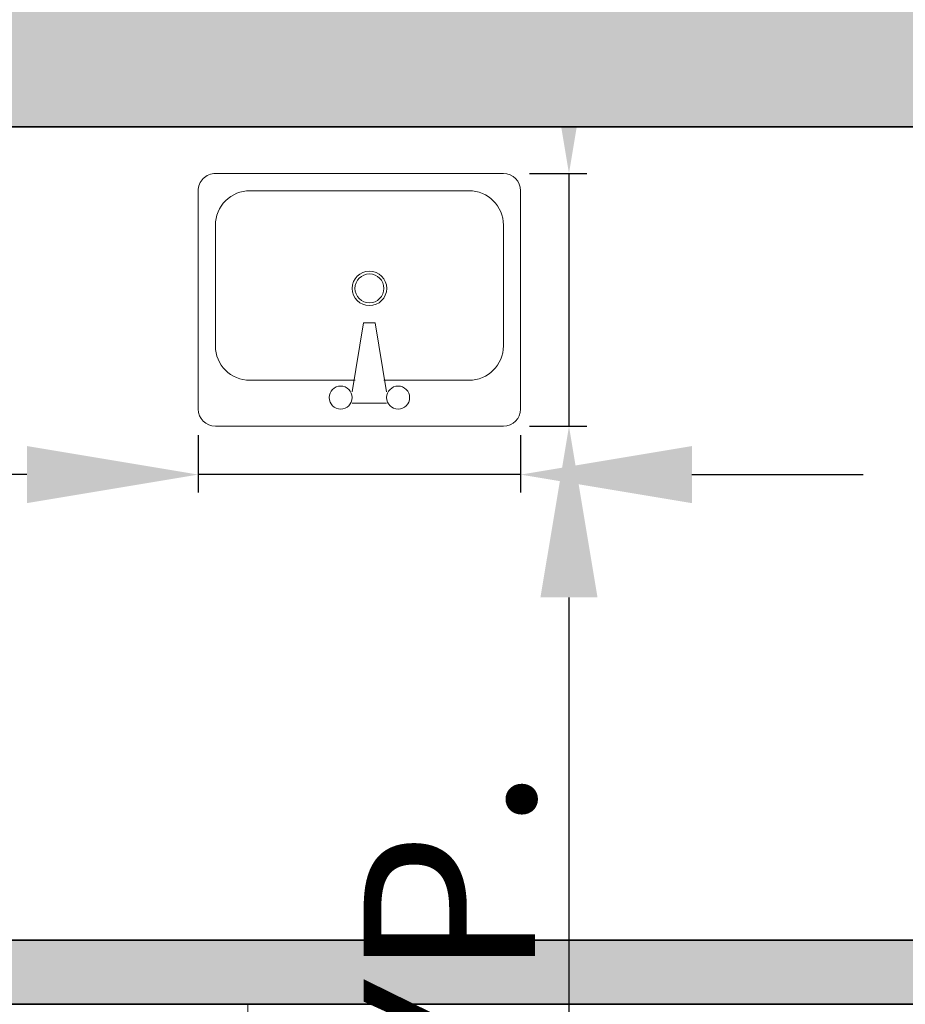
# Model space of a CAD drawing. Units: inches. Extents: x 2083 to 3317, y 1141 to 2115.
# Tile 247 of 256: x 3006 to 3068, y 1416 to 1485. Entities that reach past the tile are written whole.
import ezdxf

# ---------------------------------------------------------------- set-up
doc = ezdxf.new("R2010")
doc.units = ezdxf.units.IN
for name, color, linetype, lineweight in [('A-ANNO-DIMS', 2, 'Continuous', 18), ('A-FLOR-CASE', 8, 'Continuous', 18), ('A-FLOR-FIXT', 9, 'Continuous', 18), ('A-WALL', 7, 'Continuous', 35)]:
    doc.layers.add(name, color=color, linetype=linetype, lineweight=lineweight)
doc.layers.add('A-WALL-PATT', color=251, linetype='Continuous', lineweight=13, true_color=0x636466)
doc.styles.add('DIM_FONT', font='TXT.shx', dxfattribs={"width": 0.8})
doc.styles.get("Standard").update_dxf_attribs({"font": 'arial.ttf'})
doc.dimstyles.new('ISO-25', dxfattribs={"dimtxt": 12, "dimasz": 12, "dimexe": 1.25, "dimexo": 0.625, "dimtad": 1, "dimlunit": 3, "dimtxsty": 'Standard', "dimcen": 2.5, "dimadec": 0, "dimazin": 0, "dimtfac": 1, "dimtmove": 0, "dimatfit": 3, "dimfxl": 1, "dimarcsym": 0})

# ---------------------------------------------------------------- blocks, each defined once
blk = doc.blocks.new('A$C564A496C')
at = {"linetype": 'ByBlock'}
for p, q in [((543.2, 450), (30.7, 450)), ((0, 419.3), (0, 30.7)), ((238.5, 409.1), (299.8, 409.1)), ((573.8, 30.7), (573.8, 419.3)), ((238.5, 388.6), (258.9, 265.9)), ((279.4, 265.9), (299.8, 388.6)), ((92, 368.2), (243.6, 368.2)), ((294.7, 368.2), (481.8, 368.2)), ((30.7, 92), (30.7, 306.8)), ((543.2, 306.8), (543.2, 92)), ((258.9, 265.9), (279.4, 265.9)), ((481.8, 30.7), (92, 30.7)), ((30.7, 0), (543.2, 0))]:
    blk.add_line(p, q, dxfattribs=at)
for centre, radius in [((218, 398.9), 20.5), ((320.3, 398.9), 20.5), ((269.1, 204.5), 30.7), ((269.1, 204.5), 25.7)]:
    blk.add_circle(centre, radius, dxfattribs=at)
for centre, radius, start, end in [((30.7, 419.3), 30.7, 90, 180), ((543.2, 419.3), 30.7, 0, 90), ((92, 306.8), 61.4, 90, 180), ((481.8, 306.8), 61.4, 0, 90), ((92, 92), 61.4, 180, 270), ((481.8, 92), 61.4, 270, 0), ((30.7, 30.7), 30.7, 180, 270), ((543.2, 30.7), 30.7, 270, 0)]:
    blk.add_arc(centre, radius, start, end, dxfattribs=at)
at = {"style": 'DIM_FONT', "width": 0.8, "flags": 9}
for tag in ['YSIZE', 'XSIZE']:
    blk.add_attdef(tag, (269.1, 450), '', height=0.5, rotation=270, dxfattribs=at)
blk = doc.blocks.new('CASEWORK-96X24')
for q in [(0, 0), (24, 96)]:
    blk.add_line((0, 96), q)
blk = doc.blocks.new('*D18')
at = {"layer": 'A-ANNO-DIMS', "color": 0, "lineweight": -2, "transparency": 16777216}
for p, q in [((3018.476, 1456.156), (3018.476, 1452.142)), ((3041.068, 1456.156), (3041.068, 1452.142)), ((3006.476, 1453.392), (2828.361, 1453.392)), ((3041.068, 1453.392), (3018.476, 1453.392)), ((3053.068, 1453.392), (3065.068, 1453.392))]:
    blk.add_line(p, q, dxfattribs=at)
at = {"layer": 'A-ANNO-DIMS', "color": 0, "transparency": 16777216}
for points in [[(3006.476, 1455.392), (3006.476, 1451.392), (3018.476, 1453.392)], [(3053.068, 1455.392), (3053.068, 1451.392), (3041.068, 1453.392)]]:
    blk.add_solid(points, dxfattribs=at)
at = {"layer": 'Defpoints', "color": 0, "transparency": 16777216}
for p in [(3018.476, 1456.781), (3041.068, 1456.781), (3018.476, 1453.392)]:
    blk.add_point(p, dxfattribs=at)
at = {"layer": 'A-ANNO-DIMS', "color": 0, "transparency": 16777216, "insert": (2911.418, 1460.222), "char_height": 12, "attachment_point": 5}
blk.add_mtext('BASIN 1\'-10 1/2" TYP.', dxfattribs=at)
blk = doc.blocks.new('*D19')
at = {"layer": 'A-ANNO-DIMS', "color": 0, "lineweight": -2, "transparency": 16777216}
for p, q in [((3044.457, 1486.497), (3044.457, 1498.497)), ((3041.693, 1474.497), (3045.707, 1474.497)), ((3044.457, 1474.497), (3044.457, 1456.781)), ((3041.693, 1456.781), (3045.707, 1456.781)), ((3044.457, 1444.781), (3044.457, 1331.553))]:
    blk.add_line(p, q, dxfattribs=at)
at = {"layer": 'A-ANNO-DIMS', "color": 0, "transparency": 16777216}
for points in [[(3042.457, 1486.497), (3046.457, 1486.497), (3044.457, 1474.497)], [(3042.457, 1444.781), (3046.457, 1444.781), (3044.457, 1456.781)]]:
    blk.add_solid(points, dxfattribs=at)
at = {"layer": 'Defpoints', "color": 0, "transparency": 16777216}
for p in [(3041.068, 1474.497), (3041.068, 1456.781), (3044.457, 1456.781)]:
    blk.add_point(p, dxfattribs=at)
at = {"layer": 'A-ANNO-DIMS', "color": 0, "transparency": 16777216, "insert": (3037.627, 1382.167), "char_height": 12, "attachment_point": 5, "rotation": 90}
blk.add_mtext('1\'-5 1/2" TYP.', dxfattribs=at)

msp = doc.modelspace()

# ---------------------------------------------------------------- hatches: boundary and pattern name
at = {"layer": 'A-WALL-PATT'}
h = msp.add_hatch(color=256, dxfattribs=at)
h.dxf.hatch_style = 1
h.paths.add_polyline_path([(3126.96, 2020.761), (2748.96, 2020.761), (2604.96, 2020.761), (2226.96, 2020.761), (2226.96, 1702.761), (2466.96, 1702.761), (2466.96, 1582.761), (2418.96, 1582.761), (2418.96, 1477.761), (2226.96, 1477.761), (2226.96, 1263.261), (2544.96, 1263.261), (2544.96, 1411.761), (2604.96, 1411.761), (2685.96, 1411.761), (2685.96, 1420.761), (2604.96, 1420.761), (2604.96, 1573.761), (2604.96, 1702.761), (2604.96, 2011.761), (2748.96, 2011.761), (2748.96, 1702.761), (2862.96, 1702.761), (2862.96, 1621.761), (2871.96, 1621.761), (2871.96, 1702.761), (2883.96, 1702.761), (2883.96, 1706.939, -0.026459), (2883.96, 1711.761), (2757.96, 1711.761), (2757.96, 1807.761), (2787.96, 1807.761), (2787.96, 1812.261), (2757.96, 1812.261), (2757.96, 2011.761), (2877.96, 2011.761), (2877.96, 1812.261), (2847.96, 1812.261), (2847.96, 1807.761), (2889.836, 1807.761), (2889.836, 1812.261), (2882.46, 1812.261), (2882.46, 2011.761), (3117.96, 2011.761), (3117.96, 1812.261), (2937.836, 1812.261), (2937.836, 1807.761), (2995.71, 1807.761), (2995.71, 1796.118), (3000.21, 1796.118), (3000.21, 1807.761), (3117.96, 1807.761), (3117.96, 1711.761), (3000.21, 1711.761), (3000.21, 1760.118), (2998.573, 1760.118, -0.020711), (2995.71, 1760.118), (2995.71, 1711.761), (2931.96, 1711.761), (2931.96, 1702.761), (3126.96, 1702.761)])
h.paths.add_polyline_path([(2471.46, 2011.761), (2471.46, 1810.011), (2462.717, 1810.011), (2462.717, 1805.511), (2505.96, 1805.511), (2505.96, 1810.011), (2475.96, 1810.011), (2475.96, 2011.761), (2595.96, 2011.761), (2595.96, 1810.011), (2565.96, 1810.011), (2565.96, 1805.511), (2595.96, 1805.511), (2595.96, 1711.761), (2235.96, 1711.761), (2235.96, 1805.511), (2353.71, 1805.511), (2353.71, 1796.054), (2358.21, 1796.054), (2358.21, 1805.511), (2414.717, 1805.511), (2414.717, 1810.011), (2235.96, 1810.011), (2235.96, 2011.761)], flags=16)
h.paths.add_polyline_path([(2270.205, 1994.61), (2270.205, 1970.61), (2246.205, 1970.61), (2246.205, 1994.61)], flags=0)
edge = h.paths.add_edge_path(flags=0)
edge.add_ellipse((2332.027, 1899.798), major_axis=(-3.043, 3.043), ratio=0.168252, start_angle=-161.33217, end_angle=-156.30711, ccw=False)
edge.add_ellipse((2333.082, 1898.744), major_axis=(-1.055, 1.055), ratio=0.453532, start_angle=-123.37102, end_angle=-94.15911)
edge = h.paths.add_edge_path(flags=0)
edge.add_ellipse((2332.027, 1968.876), major_axis=(3.043, 3.043), ratio=0.168252, start_angle=18.66783, end_angle=23.69289)
edge.add_spline(control_points=[(2332.926, 1970.691), (2332.227, 1970.336), (2330.894, 1969.659), (2328.413, 1970.932), (2327.204, 1967.749), (2324.71, 1969.956), (2322.533, 1967.012), (2320.013, 1971.296), (2317.68, 1968.158), (2316.041, 1967.102), (2315.427, 1966.81)], knot_values=[0, 0, 0, 0, 2.267059, 4.324559, 6.685584, 8.878641, 11.121502, 14.300359, 17.755284, 19.732645, 19.732645, 19.732645, 19.732645], degree=3, periodic=0)
edge.add_ellipse((2332.027, 1968.876), major_axis=(3.043, 3.043), ratio=0.168252, start_angle=18.66783, end_angle=23.69289, ccw=False)
edge.add_ellipse((2333.082, 1969.931), major_axis=(1.055, 1.055), ratio=0.453532, start_angle=56.62898, end_angle=85.84089, ccw=False)
edge = h.paths.add_edge_path(flags=0)
edge.add_spline(control_points=[(2296.428, 1967.988), (2293.628, 1965.336), (2287.704, 1959.727), (2299.744, 1949.996), (2294.533, 1935.669), (2290.573, 1920.604), (2293.394, 1909.974), (2296.185, 1904.967)], knot_values=[0.099185, 0.099185, 0.099185, 0.099185, 0.345301, 0.619822, 0.982653, 1.386093, 1.810555, 1.810555, 1.810555, 1.810555], degree=3, periodic=0)
edge.add_spline(control_points=[(2296.185, 1904.967), (2297.384, 1902.619), (2298.001, 1901.949), (2298.553, 1901.468)], knot_values=[0.006246, 0.006246, 0.006246, 0.006246, 0.055476, 0.055476, 0.055476, 0.055476], degree=3, periodic=0)
edge.add_spline(control_points=[(2298.553, 1901.468), (2297.259, 1900.923), (2295.225, 1900.232), (2293.06, 1900.614), (2292.101, 1900.788), (2292.09, 1900.791)], knot_values=[0.312835, 0.312835, 0.312835, 0.312835, 0.40178, 0.474987, 0.475903, 0.475903, 0.475903, 0.475903], degree=3, periodic=0)
edge.add_arc((2292.794, 1904.664), 3.937, 215.4209, 259.69818, ccw=False)
edge.add_spline(control_points=[(2289.585, 1902.382), (2289.477, 1902.535), (2289.368, 1902.688), (2289.261, 1902.841)], knot_values=[0.102872, 0.102872, 0.102872, 0.102872, 0.116896, 0.116896, 0.116896, 0.116896], degree=3, periodic=0)
edge.add_spline(control_points=[(2289.261, 1902.841), (2288.687, 1902.55), (2287.64, 1902.02), (2285.881, 1901.874), (2283.853, 1901.504), (2281.72, 1899.711), (2278.467, 1899.493), (2276.157, 1901.883), (2272.259, 1899.804), (2267.778, 1901.843), (2262.244, 1900.184), (2257.415, 1901.782), (2254.318, 1900.726), (2253.178, 1900.337)], knot_values=[0, 0, 0, 0, 1.907977, 3.477176, 5.261074, 7.972851, 11.680248, 13.717921, 16.939592, 22.789562, 27.502503, 33.595215, 37.145618, 37.145618, 37.145618, 37.145618], degree=3, periodic=0)
edge.add_line((2253.178, 1900.337), (2250.244, 1902.841))
edge.add_line((2250.244, 1902.841), (2250.244, 1965.833))
edge.add_line((2250.244, 1965.833), (2253.178, 1968.337))
edge.add_spline(control_points=[(2253.178, 1968.337), (2254.318, 1967.948), (2257.415, 1966.892), (2262.244, 1968.49), (2267.778, 1966.831), (2271.527, 1968.537), (2273.876, 1967.828), (2274.207, 1967.728)], knot_values=[0, 0, 0, 0, 0.09018, 0.244935, 0.364644, 0.513233, 0.537855, 0.537855, 0.537855, 0.537855], degree=3, periodic=0)
edge.add_arc((2274.353, 1963.793), 3.937, 72.05113, 92.12795, ccw=False)
edge.add_arc((2281.297, 1985.23), 18.596, 252.05113, 288.56572)
edge.add_arc((2292.317, 1956.029), 12.646, 71.02679, 113.77822, ccw=False)
edge = h.paths.add_edge_path(flags=0)
edge.add_spline(control_points=[(2274.899, 1951.856), (2275.066, 1951.617), (2275.233, 1951.377), (2275.398, 1951.136)], knot_values=[1.409916, 1.409916, 1.409916, 1.409916, 1.43159, 1.43159, 1.43159, 1.43159], degree=3, periodic=0)
edge.add_spline(control_points=[(2275.398, 1951.136), (2275.792, 1950.562), (2276.179, 1949.984), (2276.546, 1949.397)], knot_values=[1.358238, 1.358238, 1.358238, 1.358238, 1.409916, 1.409916, 1.409916, 1.409916], degree=3, periodic=0)
edge.add_line((2276.546, 1949.397), (2277.437, 1947.862))
edge.add_spline(control_points=[(2277.437, 1947.862), (2276.304, 1945.673), (2274.64, 1942.427), (2274.632, 1938.094), (2272.799, 1930.852), (2274.356, 1943.897), (2275.948, 1947.923), (2276.546, 1949.397)], knot_values=[0.005632, 0.005632, 0.005632, 0.005632, 0.186014, 0.266002, 0.357087, 0.59639, 0.739732, 0.739732, 0.739732, 0.739732], degree=3, periodic=0)
edge.add_spline(control_points=[(2276.546, 1949.397), (2276.179, 1949.984), (2275.792, 1950.562), (2275.398, 1951.136)], knot_values=[1.358238, 1.358238, 1.358238, 1.358238, 1.409916, 1.409916, 1.409916, 1.409916], degree=3, periodic=0)
edge.add_spline(control_points=[(2275.398, 1951.136), (2274.943, 1950.08), (2274.208, 1948.025), (2273.935, 1944.851), (2272.469, 1937.627), (2273.466, 1945.696), (2274.701, 1951.059), (2274.899, 1951.856)], knot_values=[0.104364, 0.104364, 0.104364, 0.104364, 0.189636, 0.269624, 0.36071, 0.600013, 0.644622, 0.644622, 0.644622, 0.644622], degree=3, periodic=0)
h.paths.add_polyline_path([(2269.168, 1963.128, -0.357527), (2268.171, 1960.976, -0.092561), (2268.171, 1939.436, -0.357527), (2269.168, 1937.285, -0.357527), (2267.016, 1938.282, -0.164785), (2254.686, 1938.282, -0.357527), (2252.534, 1937.285, -0.357527), (2253.531, 1939.436, -0.092561), (2253.531, 1960.976, -0.357527), (2252.534, 1963.128, -0.357527), (2254.686, 1962.131, -0.164785), (2267.016, 1962.131, -0.357527)], flags=0)
h.paths.add_polyline_path([(2248.874, 1967.802), (2248.874, 1957.028), (2249.458, 1957.028), (2249.458, 1911.647), (2248.874, 1911.647), (2248.874, 1900.873), (2246.512, 1900.873, 0.197327), (2244.15, 1902.457), (2244.15, 1966.218, 0.197327), (2246.512, 1967.802)], flags=0)
h.paths.add_polyline_path([(2269.168, 1931.389, -0.357527), (2268.171, 1929.238, -0.092561), (2268.171, 1907.698, -0.357527), (2269.168, 1905.547, -0.357527), (2267.016, 1906.544, -0.164785), (2254.686, 1906.544, -0.357527), (2252.534, 1905.547, -0.357527), (2253.531, 1907.698, -0.092561), (2253.531, 1929.238, -0.357527), (2252.534, 1931.389, -0.357527), (2254.686, 1930.392, -0.164785), (2267.016, 1930.392, -0.357527)], flags=0)
edge = h.paths.add_edge_path(flags=0)
edge.add_spline(control_points=[(2276.197, 1906.724), (2276.168, 1909.029), (2276.114, 1913.372), (2270.598, 1924.925), (2273.905, 1919.013), (2275.922, 1916.262), (2275.475, 1912.402), (2277.258, 1910.381), (2276.696, 1908.225), (2276.646, 1906.813), (2276.618, 1906.008)], knot_values=[0, 0, 0, 0, 8.61026, 16.221274, 18.843057, 23.804898, 27.440828, 29.356102, 31.203478, 33.650687, 33.650687, 33.650687, 33.650687], degree=3, periodic=0)
edge.add_spline(control_points=[(2276.618, 1906.008), (2276.623, 1905.624), (2276.498, 1904.629), (2275.442, 1903.855), (2274.937, 1903.08), (2274.859, 1902.841)], knot_values=[0.156488, 0.156488, 0.156488, 0.156488, 0.184398, 0.231376, 0.250598, 0.250598, 0.250598, 0.250598], degree=3, periodic=0)
edge.add_line((2274.859, 1902.841), (2276.506, 1902.841))
edge.add_spline(control_points=[(2276.506, 1902.841), (2276.788, 1903.085), (2277.665, 1904.125), (2278.25, 1904.341), (2277.654, 1908.527), (2278.156, 1906.228), (2278.1, 1905.286), (2278.847, 1904.069), (2277.857, 1903.415), (2277.874, 1902.991), (2277.904, 1902.841)], knot_values=[0.059574, 0.059574, 0.059574, 0.059574, 0.080753, 0.103741, 0.16972, 0.176036, 0.207137, 0.240474, 0.262341, 0.27366, 0.27366, 0.27366, 0.27366], degree=3, periodic=0)
edge.add_line((2277.904, 1902.841), (2280.03, 1902.841))
edge.add_spline(control_points=[(2280.03, 1902.841), (2279.888, 1903.088), (2279.499, 1903.982), (2280.152, 1905.939), (2278.104, 1909.658), (2279.762, 1907.185), (2280.328, 1904.875), (2280.485, 1903.49), (2281.463, 1903.249), (2281.758, 1902.936), (2281.834, 1902.841)], knot_values=[0.013856, 0.013856, 0.013856, 0.013856, 0.034874, 0.088867, 0.107879, 0.126738, 0.158714, 0.193757, 0.217487, 0.226722, 0.226722, 0.226722, 0.226722], degree=3, periodic=0)
edge.add_spline(control_points=[(2281.834, 1902.841), (2281.788, 1902.827), (2281.647, 1902.783), (2281.396, 1902.859), (2281.088, 1902.985), (2280.721, 1903.061), (2280.333, 1903.026), (2280.125, 1902.899), (2280.03, 1902.841)], knot_values=[0, 0, 0, 0, 0.14413, 0.435517, 0.749276, 1.153046, 1.548371, 1.878348, 1.878348, 1.878348, 1.878348], degree=3, periodic=0)
edge.add_line((2280.03, 1902.841), (2277.904, 1902.841))
edge.add_spline(control_points=[(2277.904, 1902.841), (2277.893, 1902.796), (2277.865, 1902.68), (2277.607, 1902.687), (2277.274, 1902.801), (2276.838, 1902.62), (2276.584, 1902.789), (2276.506, 1902.841)], knot_values=[0, 0, 0, 0, 0.127189, 0.326199, 0.628009, 1.24357, 1.515331, 1.515331, 1.515331, 1.515331], degree=3, periodic=0)
edge.add_line((2276.506, 1902.841), (2274.859, 1902.841))
edge.add_spline(control_points=[(2274.859, 1902.841), (2274.814, 1902.899), (2274.725, 1903.013), (2274.493, 1903.119), (2274.244, 1902.961), (2273.937, 1903.185), (2273.614, 1902.983), (2273.408, 1902.883), (2273.322, 1902.841)], knot_values=[0, 0, 0, 0, 0.21843, 0.436957, 0.687977, 0.990379, 1.398396, 1.69185, 1.69185, 1.69185, 1.69185], degree=3, periodic=0)
edge.add_spline(control_points=[(2273.322, 1902.841), (2273.617, 1903.446), (2274.274, 1904.538), (2276.027, 1904.574), (2276.207, 1906.584), (2276.197, 1906.724)], knot_values=[0.012227, 0.012227, 0.012227, 0.012227, 0.059472, 0.106218, 0.134458, 0.134458, 0.134458, 0.134458], degree=3, periodic=0)
h.paths.add_polyline_path([(2270.776, 1897.79), (2270.776, 1873.79), (2246.776, 1873.79), (2246.776, 1897.79)], flags=0)
h.paths.add_polyline_path([(2353.71, 1760.005), (2353.71, 1760.054), (2358.21, 1760.054, -0.033729)], flags=0)
h.paths.add_polyline_path([(2321.819, 1737.529), (2341.995, 1737.529, -0.414214), (2343.203, 1736.321), (2343.203, 1721.021, -0.414214), (2341.995, 1719.813), (2321.819, 1719.813, -0.414214), (2320.611, 1721.021), (2320.611, 1736.321, -0.414214)], flags=0)
h.paths.add_polyline_path([(2324.235, 1736.321), (2339.579, 1736.321, -0.414214), (2341.995, 1733.905), (2341.995, 1725.45, -0.414214), (2339.579, 1723.034), (2333.681, 1723.034), (2333.845, 1722.045, -0.870646), (2335.425, 1721.826, -0.767327), (2333.923, 1721.423), (2331.291, 1721.423, -0.767327), (2329.788, 1721.826, -0.870646), (2331.368, 1722.045), (2331.533, 1723.034), (2324.235, 1723.034, -0.414214), (2321.819, 1725.45), (2321.819, 1733.905, -0.414214)], flags=0)
h.paths.add_polyline_path([(2570.484, 1928.615), (2589.684, 1928.615), (2590.169, 1928.615), (2590.169, 1904.993), (2570.484, 1904.993)], flags=0)
h.paths.add_polyline_path([(2574.447, 1927.264, -1), (2572.829, 1927.264, -1)], flags=0)
h.paths.add_polyline_path([(2573.09, 1926.941), (2573.925, 1927.776), (2574.148, 1927.553), (2573.313, 1926.718)], flags=0)
h.paths.add_polyline_path([(2578.779, 1919.73, -1), (2571.592, 1919.73, -1)], flags=0)
h.paths.add_polyline_path([(2578.385, 1919.73, -1), (2571.985, 1919.73, -1)], flags=0)
h.paths.add_polyline_path([(2331.596, 1729.476, -1), (2333.618, 1729.476, -1)], flags=0)
h.paths.add_polyline_path([(2578.034, 1927.264, -1), (2576.416, 1927.264, -1)], flags=0)
h.paths.add_polyline_path([(2576.689, 1927.531), (2576.912, 1927.754), (2577.747, 1926.919), (2577.524, 1926.696)], flags=0)
h.paths.add_polyline_path([(2578.139, 1909.86, -1), (2572.232, 1909.86, -1)], flags=0)
h.paths.add_polyline_path([(2577.745, 1909.86, -1), (2572.625, 1909.86, -1)], flags=0)
h.paths.add_polyline_path([(2583.798, 1927.264, -1), (2582.179, 1927.264, -1)], flags=0)
h.paths.add_polyline_path([(2582.719, 1927.754), (2583.554, 1926.919), (2583.331, 1926.696), (2582.496, 1927.531)], flags=0)
h.paths.add_polyline_path([(2582.496, 1927.531), (2582.719, 1927.754), (2583.554, 1926.919), (2583.331, 1926.696)], flags=0)
h.paths.add_polyline_path([(2587.739, 1920.53, -1), (2581.832, 1920.53, -1)], flags=0)
h.paths.add_polyline_path([(2587.345, 1920.53, -1), (2582.225, 1920.53, -1)], flags=0)
h.paths.add_polyline_path([(2587.385, 1927.264, -1), (2585.766, 1927.264, -1)], flags=0)
h.paths.add_polyline_path([(2586.082, 1926.98), (2586.917, 1927.815), (2587.14, 1927.593), (2586.305, 1926.758)], flags=0)
h.paths.add_polyline_path([(2588.379, 1910.66, -1), (2581.192, 1910.66, -1)], flags=0)
h.paths.add_polyline_path([(2587.985, 1910.66, -1), (2581.585, 1910.66, -1)], flags=0)
h.paths.add_polyline_path([(2417.168, 1729.478), (2437.344, 1729.478, -0.414214), (2438.552, 1728.27), (2438.552, 1712.969, -0.414214), (2437.344, 1711.761), (2417.168, 1711.761, -0.414214), (2415.96, 1712.969), (2415.96, 1728.27, -0.414214)], flags=0)
h.paths.add_polyline_path([(2419.584, 1728.27), (2434.928, 1728.27, -0.414214), (2437.344, 1725.854), (2437.344, 1717.398, -0.414214), (2434.928, 1714.983), (2429.029, 1714.983), (2429.194, 1713.994, -0.870646), (2430.774, 1713.775, -0.767327), (2429.271, 1713.372), (2426.64, 1713.372, -0.767327), (2425.137, 1713.775, -0.870646), (2426.717, 1713.994), (2426.882, 1714.983), (2419.584, 1714.983, -0.414214), (2417.168, 1717.398), (2417.168, 1725.854, -0.414214)], flags=0)
h.paths.add_polyline_path([(2419.584, 1728.27), (2434.928, 1728.27, -0.414214), (2437.344, 1725.854), (2437.344, 1717.398, -0.414214), (2434.928, 1714.983), (2429.029, 1714.983), (2428.358, 1719.009), (2427.553, 1719.009), (2426.882, 1714.983), (2419.584, 1714.983, -0.414214), (2417.168, 1717.398), (2417.168, 1725.854, -0.414214)], flags=0)
h.paths.add_polyline_path([(2426.944, 1721.425, -1), (2428.967, 1721.425, -1)], flags=0)
h.paths.add_polyline_path([(2475.96, 1702.761), (2595.96, 1702.761), (2595.96, 1582.761), (2475.96, 1582.761)], flags=16)
h.paths.add_polyline_path([(2427.96, 1573.761), (2595.96, 1573.761), (2595.96, 1468.761), (2595.96, 1420.761), (2384.46, 1420.761), (2384.46, 1468.761), (2427.96, 1468.761)], flags=16)
h.paths.add_polyline_path([(2379.96, 1468.761), (2379.96, 1420.761), (2235.96, 1420.761), (2235.96, 1468.761)], flags=16)
h.paths.add_polyline_path([(2317.816, 1466.696), (2337.992, 1466.696, -0.414214), (2339.2, 1465.488), (2339.2, 1450.187, -0.414214), (2337.992, 1448.979), (2317.816, 1448.979, -0.414214), (2316.608, 1450.187), (2316.608, 1465.488, -0.414214)], flags=0)
h.paths.add_polyline_path([(2320.232, 1465.488), (2335.576, 1465.488, -0.414214), (2337.992, 1463.072), (2337.992, 1454.616, -0.414214), (2335.576, 1452.2), (2329.677, 1452.2), (2329.842, 1451.212, -0.870646), (2331.422, 1450.992, -0.767327), (2329.92, 1450.59), (2327.288, 1450.59, -0.767327), (2325.785, 1450.992, -0.870646), (2327.365, 1451.212), (2327.53, 1452.2), (2320.232, 1452.2, -0.414214), (2317.816, 1454.616), (2317.816, 1463.072, -0.414214)], flags=0)
h.paths.add_polyline_path([(2320.232, 1465.488), (2335.576, 1465.488, -0.414214), (2337.992, 1463.072), (2337.992, 1454.616, -0.414214), (2335.576, 1452.2), (2329.677, 1452.2), (2329.006, 1456.227), (2328.201, 1456.227), (2327.53, 1452.2), (2320.232, 1452.2, -0.414214), (2317.816, 1454.616), (2317.816, 1463.072, -0.414214)], flags=0)
h.paths.add_polyline_path([(2327.593, 1458.643, -1), (2329.615, 1458.643, -1)], flags=0)
h.paths.add_polyline_path([(2244.412, 1433.34), (2241.921, 1433.34, -0.414214), (2240.018, 1435.244), (2240.018, 1440.953, -0.414211), (2241.921, 1442.856), (2244.412, 1442.856, -1.976472)], flags=0)
h.paths.add_polyline_path([(2245.357, 1434.398, -0.414214), (2245.357, 1441.799, -2.144098)], flags=0)
h.paths.add_polyline_path([(2535.96, 1416.261), (2535.96, 1272.261), (2235.96, 1272.261), (2235.96, 1416.261)], flags=16)
h.paths.add_polyline_path([(2260.12, 1384.293), (2260.12, 1362.039), (2237.865, 1362.039), (2237.865, 1384.293)], flags=0)
edge = h.paths.add_edge_path(flags=0)
edge.add_line((2318.252, 1362.093), (2318.146, 1362.001))
edge.add_ellipse((2317.445, 1360.431), major_axis=(2.822, 2.822), ratio=0.168252, start_angle=18.66783, end_angle=20.94813, ccw=False)
edge.add_ellipse((2318.423, 1361.409), major_axis=(0.978, 0.978), ratio=0.453532, start_angle=56.62898, end_angle=70.2262, ccw=False)
edge = h.paths.add_edge_path(flags=0)
edge.add_line((2319.107, 1295.571), (2319.015, 1295.677))
edge.add_ellipse((2317.445, 1296.378), major_axis=(-2.822, 2.822), ratio=0.168252, start_angle=-161.33217, end_angle=-159.05187, ccw=False)
edge.add_ellipse((2318.423, 1295.4), major_axis=(-0.978, 0.978), ratio=0.453532, start_angle=-123.37102, end_angle=-109.7738)
edge = h.paths.add_edge_path(flags=0)
edge.add_spline(control_points=[(2284.21, 1301.17), (2284.581, 1300.445), (2284.891, 1299.892), (2285.16, 1299.461)], knot_values=[0.039066, 0.039066, 0.039066, 0.039066, 0.055476, 0.055476, 0.055476, 0.055476], degree=3, periodic=0)
edge.add_line((2285.16, 1299.461), (2284.21, 1301.17))
edge = h.paths.add_edge_path(flags=0)
edge.add_line((2280.412, 1297.298), (2283.37, 1297.036))
edge.add_line((2283.37, 1297.036), (2286.406, 1297.926))
edge.add_spline(control_points=[(2286.406, 1297.926), (2285.305, 1297.463), (2284.345, 1297.129), (2283.37, 1297.036)], knot_values=[0.394369, 0.394369, 0.394369, 0.394369, 0.475903, 0.475903, 0.475903, 0.475903], degree=3, periodic=0)
edge.add_spline(control_points=[(2283.37, 1297.036), (2283.281, 1297.028), (2282.316, 1296.957), (2281.313, 1297.134), (2280.423, 1297.296), (2280.412, 1297.298)], knot_values=[0.312835, 0.312835, 0.312835, 0.312835, 0.320246, 0.393453, 0.394369, 0.394369, 0.394369, 0.394369], degree=3, periodic=0)
edge = h.paths.add_edge_path(flags=0)
edge.add_line((2284.436, 1359.607), (2280.446, 1355.328))
edge.add_line((2280.446, 1355.328), (2279.58, 1351.018))
edge.add_line((2279.58, 1351.018), (2282.413, 1346.58))
edge.add_spline(control_points=[(2282.413, 1346.58), (2283.153, 1345.589), (2284.253, 1344.029), (2284.801, 1342.387), (2284.935, 1341.806)], knot_values=[1.240098, 1.240098, 1.240098, 1.240098, 1.332892, 1.382712, 1.382712, 1.382712, 1.382712], degree=3, periodic=0)
edge.add_spline(control_points=[(2284.935, 1341.806), (2285.319, 1340.141), (2285.233, 1338.409), (2284.91, 1336.654)], knot_values=[1.097484, 1.097484, 1.097484, 1.097484, 1.240098, 1.240098, 1.240098, 1.240098], degree=3, periodic=0)
edge.add_spline(control_points=[(2284.91, 1336.654), (2284.587, 1334.899), (2284.027, 1333.12), (2283.463, 1331.361)], knot_values=[0.95487, 0.95487, 0.95487, 0.95487, 1.097484, 1.097484, 1.097484, 1.097484], degree=3, periodic=0)
edge.add_line((2283.463, 1331.361), (2281.89, 1326.153))
edge.add_line((2281.89, 1326.153), (2280.756, 1321.056))
edge.add_line((2280.756, 1321.056), (2280.299, 1316.002))
edge.add_line((2280.299, 1316.002), (2280.716, 1310.95))
edge.add_line((2280.716, 1310.95), (2282.028, 1305.972))
edge.add_line((2282.028, 1305.972), (2284.21, 1301.17))
edge.add_spline(control_points=[(2284.21, 1301.17), (2283.341, 1302.73), (2282.612, 1304.336), (2282.028, 1305.972)], knot_values=[0.099185, 0.099185, 0.099185, 0.099185, 0.241799, 0.241799, 0.241799, 0.241799], degree=3, periodic=0)
edge.add_spline(control_points=[(2282.028, 1305.972), (2281.444, 1307.608), (2281.005, 1309.273), (2280.716, 1310.95)], knot_values=[0.241799, 0.241799, 0.241799, 0.241799, 0.384413, 0.384413, 0.384413, 0.384413], degree=3, periodic=0)
edge.add_spline(control_points=[(2280.716, 1310.95), (2280.433, 1312.588), (2280.289, 1314.277), (2280.299, 1315.962), (2280.299, 1316.002)], knot_values=[0.384413, 0.384413, 0.384413, 0.384413, 0.523647, 0.527028, 0.527028, 0.527028, 0.527028], degree=3, periodic=0)
edge.add_spline(control_points=[(2280.299, 1316.002), (2280.312, 1317.687), (2280.478, 1319.368), (2280.756, 1321.056)], knot_values=[0.527028, 0.527028, 0.527028, 0.527028, 0.669642, 0.669642, 0.669642, 0.669642], degree=3, periodic=0)
edge.add_spline(control_points=[(2280.756, 1321.056), (2281.035, 1322.744), (2281.426, 1324.44), (2281.89, 1326.153)], knot_values=[0.669642, 0.669642, 0.669642, 0.669642, 0.812256, 0.812256, 0.812256, 0.812256], degree=3, periodic=0)
edge.add_spline(control_points=[(2281.89, 1326.153), (2282.264, 1327.533), (2282.788, 1329.262), (2283.353, 1331.018), (2283.463, 1331.361)], knot_values=[0.812256, 0.812256, 0.812256, 0.812256, 0.927087, 0.95487, 0.95487, 0.95487, 0.95487], degree=3, periodic=0)
edge.add_line((2283.463, 1331.361), (2284.91, 1336.654))
edge.add_line((2284.91, 1336.654), (2284.935, 1341.806))
edge.add_line((2284.935, 1341.806), (2282.413, 1346.58))
edge.add_spline(control_points=[(2282.413, 1346.58), (2281.275, 1348.104), (2280.078, 1349.57), (2279.58, 1351.018)], knot_values=[1.382712, 1.382712, 1.382712, 1.382712, 1.525326, 1.525326, 1.525326, 1.525326], degree=3, periodic=0)
edge.add_spline(control_points=[(2279.58, 1351.018), (2279.443, 1351.415), (2279.136, 1352.857), (2279.735, 1354.29), (2280.446, 1355.328)], knot_values=[1.525326, 1.525326, 1.525326, 1.525326, 1.564439, 1.667941, 1.667941, 1.667941, 1.667941], degree=3, periodic=0)
edge.add_spline(control_points=[(2280.446, 1355.328), (2281.426, 1356.758), (2282.931, 1358.183), (2284.436, 1359.607)], knot_values=[1.667941, 1.667941, 1.667941, 1.667941, 1.810555, 1.810555, 1.810555, 1.810555], degree=3, periodic=0)
edge.add_arc((2280.623, 1348.518), 11.726, 71.02679, 113.77822)
edge.add_arc((2270.405, 1375.595), 17.244, 252.05113, 288.56572, ccw=False)
edge.add_arc((2263.966, 1355.718), 3.651, 72.05113, 92.12795)
edge.add_arc((2263.966, 1355.718), 3.651, 92.12795, 177.98513)
edge.add_spline(control_points=[(2260.318, 1355.846), (2260.26, 1354.221), (2260.551, 1350.187), (2262.999, 1346.766), (2264.473, 1344.649)], knot_values=[1.43159, 1.43159, 1.43159, 1.43159, 1.564144, 1.770695, 1.770695, 1.770695, 1.770695], degree=3, periodic=0)
edge.add_line((2264.473, 1344.649), (2264.936, 1343.983))
edge.add_spline(control_points=[(2263.801, 1340.248), (2263.843, 1340.514), (2264.067, 1341.756), (2264.513, 1343.002), (2264.935, 1343.981)], knot_values=[0.53657, 0.53657, 0.53657, 0.53657, 0.559349, 0.644622, 0.644622, 0.644622, 0.644622], degree=3, periodic=0)
edge.add_spline(control_points=[(2264.935, 1343.981), (2265.118, 1343.715), (2265.299, 1343.448), (2265.477, 1343.179)], knot_values=[1.384077, 1.384077, 1.384077, 1.384077, 1.409916, 1.409916, 1.409916, 1.409916], degree=3, periodic=0)
edge.add_spline(control_points=[(2265.477, 1343.179), (2265.655, 1342.911), (2265.829, 1342.641), (2265.999, 1342.369)], knot_values=[1.358238, 1.358238, 1.358238, 1.358238, 1.384077, 1.384077, 1.384077, 1.384077], degree=3, periodic=0)
edge.add_line((2265.999, 1342.369), (2266.826, 1340.946))
edge.add_spline(control_points=[(2266.826, 1340.946), (2268.894, 1337.09), (2271.398, 1325.843), (2270.516, 1310.569), (2275.919, 1301.861), (2277.79, 1299.199)], knot_values=[0.116896, 0.116896, 0.116896, 0.116896, 0.472987, 1.050969, 1.313793, 1.313793, 1.313793, 1.313793], degree=3, periodic=0)
edge.add_spline(control_points=[(2277.79, 1299.199), (2277.839, 1299.128), (2277.889, 1299.057), (2277.94, 1298.987)], knot_values=[0.109884, 0.109884, 0.109884, 0.109884, 0.116896, 0.116896, 0.116896, 0.116896], degree=3, periodic=0)
edge.add_line((2277.94, 1298.987), (2277.789, 1299.199))
edge.add_spline(control_points=[(2277.789, 1299.199), (2277.257, 1298.929), (2276.286, 1298.438), (2275.039, 1298.334), (2274.383, 1298.239), (2274.215, 1298.209)], knot_values=[33.12187, 33.12187, 33.12187, 33.12187, 35.029056, 36.598255, 37.144827, 37.144827, 37.144827, 37.144827], degree=3, periodic=0)
edge.add_line((2274.215, 1298.209), (2273.073, 1297.893))
edge.add_spline(control_points=[(2273.073, 1297.893), (2272.323, 1297.58), (2271.039, 1296.511), (2269.248, 1296.226), (2268.423, 1296.375)], knot_values=[26.532584, 26.532584, 26.532584, 26.532584, 29.198919, 31.839101, 31.839101, 31.839101, 31.839101], degree=3, periodic=0)
edge.add_line((2268.423, 1296.375), (2263.879, 1297.458))
edge.add_spline(control_points=[(2263.879, 1297.458), (2263.556, 1297.359), (2261.86, 1296.839), (2260.239, 1297.282), (2258.933, 1297.516)], knot_values=[15.919551, 15.919551, 15.919551, 15.919551, 16.939592, 21.226067, 21.226067, 21.226067, 21.226067], degree=3, periodic=0)
edge.add_line((2258.933, 1297.516), (2254.055, 1297.329))
edge.add_spline(control_points=[(2254.055, 1297.329), (2253.756, 1297.296), (2252.114, 1297.165), (2250.462, 1297.544), (2249.13, 1297.668)], knot_values=[5.306517, 5.306517, 5.306517, 5.306517, 6.276435, 10.613034, 10.613034, 10.613034, 10.613034], degree=3, periodic=0)
edge.add_line((2249.13, 1297.668), (2244.332, 1296.878))
edge.add_line((2244.332, 1296.878), (2241.611, 1299.199))
edge.add_line((2241.611, 1299.199), (2241.611, 1357.609))
edge.add_line((2241.611, 1357.609), (2244.332, 1359.931))
edge.add_line((2244.332, 1359.931), (2252.729, 1359.543))
edge.add_spline(control_points=[(2252.729, 1359.543), (2252.871, 1359.546), (2253.306, 1359.548), (2253.74, 1359.514), (2254.032, 1359.482)], knot_values=[0.233291, 0.233291, 0.233291, 0.233291, 0.244935, 0.268927, 0.268927, 0.268927, 0.268927], degree=3, periodic=0)
edge.add_line((2254.032, 1359.482), (2259.587, 1359.416))
edge.add_spline(control_points=[(2259.587, 1359.416), (2260.677, 1359.629), (2262.073, 1359.897), (2263.524, 1359.459), (2263.83, 1359.366)], knot_values=[0.422516, 0.422516, 0.422516, 0.422516, 0.513233, 0.537855, 0.537855, 0.537855, 0.537855], degree=3, periodic=0)
edge.add_arc((2263.966, 1355.718), 3.651, 72.05113, 92.12795, ccw=False)
edge.add_arc((2270.405, 1375.595), 17.244, 252.05113, 288.56572)
edge.add_arc((2280.623, 1348.518), 11.726, 71.02679, 113.77822, ccw=False)
h.paths.add_polyline_path([(2240.341, 1359.435), (2240.341, 1349.444), (2240.882, 1349.444), (2240.882, 1307.365), (2240.341, 1307.365), (2240.341, 1297.374), (2238.15, 1297.374, 0.197327), (2235.96, 1298.843), (2235.96, 1357.966, 0.197327), (2238.15, 1359.435)], flags=0)
h.paths.add_polyline_path([(2259.158, 1355.101, -0.357527), (2258.233, 1353.106, -0.092561), (2258.233, 1333.133, -0.357527), (2259.158, 1331.138, -0.357527), (2257.163, 1332.062, -0.164785), (2245.729, 1332.062, -0.357527), (2243.735, 1331.138, -0.357527), (2244.659, 1333.133, -0.092561), (2244.659, 1353.106, -0.357527), (2243.735, 1355.101, -0.357527), (2245.729, 1354.176, -0.164785), (2257.163, 1354.176, -0.357527)], flags=0)
edge = h.paths.add_edge_path(flags=0)
edge.add_line((2265.999, 1342.369), (2266.826, 1340.946))
edge.add_line((2266.826, 1340.946), (2265.308, 1337.814))
edge.add_line((2265.308, 1337.814), (2264.358, 1334.653))
edge.add_line((2264.358, 1334.653), (2264.262, 1333.8))
edge.add_spline(control_points=[(2264.262, 1333.8), (2264.208, 1333.187), (2264.162, 1332.366), (2264.007, 1331.414), (2263.969, 1331.202)], knot_values=[0.464444, 0.464444, 0.464444, 0.464444, 0.516691, 0.531608, 0.531608, 0.531608, 0.531608], degree=3, periodic=0)
edge.add_spline(control_points=[(2263.969, 1331.202), (2263.775, 1330.119), (2263.424, 1328.791), (2263.257, 1328.531), (2263.234, 1328.515)], knot_values=[0.372682, 0.372682, 0.372682, 0.372682, 0.44885, 0.464444, 0.464444, 0.464444, 0.464444], degree=3, periodic=0)
edge.add_spline(control_points=[(2263.234, 1328.515), (2263.096, 1328.42), (2263.131, 1329.301), (2263.275, 1330.616)], knot_values=[0.280919, 0.280919, 0.280919, 0.280919, 0.372682, 0.372682, 0.372682, 0.372682], degree=3, periodic=0)
edge.add_spline(control_points=[(2263.275, 1330.616), (2263.419, 1331.93), (2263.672, 1333.677), (2263.97, 1335.315)], knot_values=[0.189157, 0.189157, 0.189157, 0.189157, 0.280919, 0.280919, 0.280919, 0.280919], degree=3, periodic=0)
edge.add_spline(control_points=[(2263.97, 1335.315), (2264.1, 1336.032), (2264.419, 1337.622), (2264.755, 1338.864), (2264.947, 1339.491)], knot_values=[0.097394, 0.097394, 0.097394, 0.097394, 0.137578, 0.189157, 0.189157, 0.189157, 0.189157], degree=3, periodic=0)
edge.add_spline(control_points=[(2264.947, 1339.491), (2265.29, 1340.606), (2265.644, 1341.494), (2265.999, 1342.369)], knot_values=[0.005632, 0.005632, 0.005632, 0.005632, 0.097394, 0.097394, 0.097394, 0.097394], degree=3, periodic=0)
h.paths.add_polyline_path([(2259.158, 1325.671, -0.357527), (2258.233, 1323.676, -0.092561), (2258.233, 1303.703, -0.357527), (2259.158, 1301.708, -0.357527), (2257.163, 1302.633, -0.164785), (2245.729, 1302.633, -0.357527), (2243.735, 1301.708, -0.357527), (2244.659, 1303.703, -0.092561), (2244.659, 1323.676, -0.357527), (2243.735, 1325.671, -0.357527), (2245.729, 1324.747, -0.164785), (2257.163, 1324.747, -0.357527)], flags=0)
edge = h.paths.add_edge_path(flags=0)
edge.add_spline(control_points=[(2261.709, 1317.311), (2261.679, 1317.418), (2261.762, 1317.389), (2262.491, 1316.09), (2262.962, 1315.301)], knot_values=[14.955861, 14.955861, 14.955861, 14.955861, 16.221274, 18.694826, 18.694826, 18.694826, 18.694826], degree=3, periodic=0)
edge.add_spline(control_points=[(2262.962, 1315.301), (2262.99, 1315.254), (2263.702, 1314.067), (2264.349, 1313.127), (2264.73, 1312.164)], knot_values=[18.694826, 18.694826, 18.694826, 18.694826, 18.843057, 22.433791, 22.433791, 22.433791, 22.433791], degree=3, periodic=0)
edge.add_spline(control_points=[(2264.73, 1312.164), (2264.876, 1311.796), (2265.177, 1310.77), (2265.143, 1309.559), (2265.248, 1308.824)], knot_values=[22.433791, 22.433791, 22.433791, 22.433791, 23.804898, 26.172756, 26.172756, 26.172756, 26.172756], degree=3, periodic=0)
edge.add_line((2265.248, 1308.824), (2265.851, 1307.172))
edge.add_spline(control_points=[(2265.851, 1307.172), (2266.065, 1306.822), (2266.384, 1306.332), (2266.424, 1305.781), (2266.42, 1305.611)], knot_values=[28.062562, 28.062562, 28.062562, 28.062562, 29.356102, 29.911721, 29.911721, 29.911721, 29.911721], degree=3, periodic=0)
edge.add_spline(control_points=[(2266.42, 1305.611), (2266.416, 1305.433), (2266.394, 1305.25), (2266.365, 1305.066)], knot_values=[29.911721, 29.911721, 29.911721, 29.911721, 30.497837, 30.497837, 30.497837, 30.497837], degree=3, periodic=0)
edge.add_line((2266.365, 1305.066), (2266.066, 1302.136))
edge.add_spline(control_points=[(2266.066, 1302.136), (2266.071, 1301.78), (2265.998, 1301.2), (2265.663, 1300.759), (2265.509, 1300.586)], knot_values=[0.156488, 0.156488, 0.156488, 0.156488, 0.184398, 0.203543, 0.203543, 0.203543, 0.203543], degree=3, periodic=0)
edge.add_line((2265.509, 1300.586), (2264.435, 1299.199))
edge.add_line((2264.435, 1299.199), (2265.962, 1299.199))
edge.add_line((2265.962, 1299.199), (2267.336, 1301.175))
edge.add_line((2267.336, 1301.175), (2267.312, 1301.986))
edge.add_spline(control_points=[(2267.312, 1301.986), (2267.261, 1302.862), (2267.16, 1303.737), (2267.271, 1303.326)], knot_values=[0.126229, 0.126229, 0.126229, 0.126229, 0.166617, 0.166617, 0.166617, 0.166617], degree=3, periodic=0)
edge.add_spline(control_points=[(2267.271, 1303.326), (2267.28, 1303.294), (2267.31, 1303.175), (2267.373, 1302.884), (2267.406, 1302.683), (2267.418, 1302.601)], knot_values=[0.166617, 0.166617, 0.166617, 0.166617, 0.16972, 0.176036, 0.180765, 0.180765, 0.180765, 0.180765], degree=3, periodic=0)
edge.add_spline(control_points=[(2267.744, 1300.988), (2267.688, 1301.151), (2267.481, 1301.657), (2267.484, 1302.145), (2267.418, 1302.601)], knot_values=[0.180765, 0.180765, 0.180765, 0.180765, 0.193767, 0.220139, 0.220139, 0.220139, 0.220139], degree=3, periodic=0)
edge.add_line((2267.418, 1302.601), (2267.744, 1300.988))
edge.add_spline(control_points=[(2267.744, 1300.988), (2267.832, 1300.732), (2267.932, 1300.31), (2267.555, 1299.975), (2267.429, 1299.829)], knot_values=[0.220139, 0.220139, 0.220139, 0.220139, 0.240474, 0.25489, 0.25489, 0.25489, 0.25489], degree=3, periodic=0)
edge.add_line((2267.429, 1299.829), (2267.258, 1299.199))
edge.add_line((2267.258, 1299.199), (2269.23, 1299.199))
edge.add_spline(control_points=[(2269.23, 1299.199), (2269.099, 1299.429), (2268.843, 1300.016), (2269.012, 1300.916), (2268.947, 1301.661)], knot_values=[0.013856, 0.013856, 0.013856, 0.013856, 0.034874, 0.067073, 0.067073, 0.067073, 0.067073], degree=3, periodic=0)
edge.add_line((2268.947, 1301.661), (2268.432, 1303.603))
edge.add_spline(control_points=[(2268.432, 1303.603), (2268.176, 1304.192), (2267.596, 1305.251), (2268.041, 1304.623), (2268.251, 1304.282)], knot_values=[0.090155, 0.090155, 0.090155, 0.090155, 0.107879, 0.120289, 0.120289, 0.120289, 0.120289], degree=3, periodic=0)
edge.add_spline(control_points=[(2268.251, 1304.282), (2268.361, 1304.105), (2269.058, 1302.918), (2269.383, 1301.59), (2269.521, 1300.776), (2269.575, 1300.556)], knot_values=[0.120289, 0.120289, 0.120289, 0.120289, 0.126738, 0.158714, 0.173506, 0.173506, 0.173506, 0.173506], degree=3, periodic=0)
edge.add_line((2269.575, 1300.556), (2270.686, 1299.421))
edge.add_spline(control_points=[(2270.686, 1299.421), (2270.767, 1299.357), (2270.838, 1299.281), (2270.903, 1299.199)], knot_values=[0.21816, 0.21816, 0.21816, 0.21816, 0.226722, 0.226722, 0.226722, 0.226722], degree=3, periodic=0)
edge.add_line((2270.937, 1299.193), (2270.903, 1299.199))
edge.add_spline(control_points=[(2270.903, 1299.199), (2270.86, 1299.186), (2270.73, 1299.146), (2270.496, 1299.216), (2270.272, 1299.308), (2270.121, 1299.348), (2270.063, 1299.36)], knot_values=[0.939174, 0.939174, 0.939174, 0.939174, 1.083304, 1.374691, 1.68845, 1.878348, 1.878348, 1.878348, 1.878348], degree=3, periodic=0)
edge.add_line((2270.063, 1299.36), (2269.23, 1299.199))
edge.add_line((2269.23, 1299.199), (2267.258, 1299.199))
edge.add_spline(control_points=[(2267.258, 1299.199), (2267.248, 1299.157), (2267.223, 1299.05), (2266.984, 1299.057), (2266.809, 1299.116), (2266.677, 1299.109), (2266.637, 1299.105)], knot_values=[0.757665, 0.757665, 0.757665, 0.757665, 0.884854, 1.083864, 1.385675, 1.515331, 1.515331, 1.515331, 1.515331], degree=3, periodic=0)
edge.add_spline(control_points=[(2266.637, 1299.105), (2266.485, 1299.089), (2266.236, 1299.017), (2266.035, 1299.151), (2265.962, 1299.199)], knot_values=[0, 0, 0, 0, 0.485905, 0.757665, 0.757665, 0.757665, 0.757665], degree=3, periodic=0)
edge.add_line((2265.962, 1299.199), (2264.435, 1299.199))
edge.add_line((2264.435, 1299.199), (2263.858, 1299.367))
edge.add_spline(control_points=[(2263.858, 1299.367), (2263.819, 1299.371), (2263.78, 1299.386), (2263.74, 1299.402)], knot_values=[0.845925, 0.845925, 0.845925, 0.845925, 0.978627, 0.978627, 0.978627, 0.978627], degree=3, periodic=0)
edge.add_line((2263.722, 1299.396), (2263.01, 1299.199))
edge.add_spline(control_points=[(2263.01, 1299.199), (2263.246, 1299.683), (2263.506, 1300.128), (2263.873, 1300.408)], knot_values=[0.012227, 0.012227, 0.012227, 0.012227, 0.052971, 0.052971, 0.052971, 0.052971], degree=3, periodic=0)
edge.add_spline(control_points=[(2263.873, 1300.408), (2263.932, 1300.453), (2264.084, 1300.553), (2264.255, 1300.624), (2264.36, 1300.665)], knot_values=[0.052971, 0.052971, 0.052971, 0.052971, 0.059472, 0.069086, 0.069086, 0.069086, 0.069086], degree=3, periodic=0)
edge.add_line((2264.36, 1300.665), (2265.142, 1301.078))
edge.add_line((2265.142, 1301.078), (2265.676, 1302.8))
edge.add_line((2265.676, 1302.8), (2265.541, 1305.704))
edge.add_line((2265.541, 1305.704), (2264.803, 1309.328))
edge.add_line((2264.803, 1309.328), (2263.041, 1314.092))
edge.add_spline(control_points=[(2263.041, 1314.092), (2262.384, 1315.671), (2261.796, 1316.998), (2261.709, 1317.311)], knot_values=[11.216896, 11.216896, 11.216896, 11.216896, 14.955861, 14.955861, 14.955861, 14.955861], degree=3, periodic=0)
h.paths.add_polyline_path([(2871.96, 1416.261), (2895.91, 1416.261), (2895.91, 1420.761), (2871.96, 1420.761), (2871.96, 1501.761), (2862.96, 1501.761), (2862.96, 1420.761), (2805.96, 1420.761), (2805.96, 1411.761), (2862.96, 1411.761), (2862.96, 1263.261), (3126.96, 1263.261), (3126.96, 1411.761), (3126.96, 1486.761), (2943.96, 1486.761), (2943.96, 1477.761), (2967.86, 1477.761), (2967.86, 1420.761), (2943.91, 1420.761), (2943.91, 1416.261), (3117.96, 1416.261), (3117.96, 1420.761), (2972.36, 1420.761), (2972.36, 1477.761), (3117.96, 1477.761), (3117.96, 1420.761), (3117.96, 1272.261), (2871.96, 1272.261)], flags=0)
h.paths.add_polyline_path([(2457.126, 1485.943), (2527.603, 1485.943), (2527.603, 1537.636), (2457.126, 1537.636)], flags=8)
h.paths.add_polyline_path([(2481.005, 1609.982), (2590.766, 1609.982), (2590.766, 1682.003), (2481.005, 1682.003)], flags=8)
h.paths.add_polyline_path([(2483.085, 1729.127), (2553.562, 1729.127), (2553.562, 1780.82), (2483.085, 1780.82)], flags=8)
h = msp.add_hatch(color=256, dxfattribs=at)
h.dxf.hatch_style = 1
h.paths.add_polyline_path([(3126.96, 1486.761), (2943.96, 1486.761), (2943.96, 1477.761), (2967.86, 1477.761), (2967.86, 1420.761), (2943.91, 1420.761), (2943.91, 1416.261), (3117.96, 1416.261), (3117.96, 1420.761), (2972.36, 1420.761), (2972.36, 1477.761), (3117.96, 1477.761), (3117.96, 1420.761), (3117.96, 1272.261), (2871.96, 1272.261), (2871.96, 1416.261), (2895.91, 1416.261), (2895.91, 1420.761), (2871.96, 1420.761), (2871.96, 1501.761), (2862.96, 1501.761), (2862.96, 1420.761), (2805.96, 1420.761), (2805.96, 1411.761), (2862.96, 1411.761), (2862.96, 1263.261), (3126.96, 1263.261), (3126.96, 1411.761)])

# ---------------------------------------------------------------- linework, layer by layer
at = {"layer": 'A-WALL'}
for p, q in [((2972.36, 1477.761), (3117.96, 1477.761)), ((2972.36, 1420.761), (3117.96, 1420.761)), ((2943.91, 1416.261), (3117.96, 1416.261))]:
    msp.add_line(p, q, dxfattribs=at)

# ---------------------------------------------------------------- block references
at = {"layer": 'A-FLOR-CASE', "rotation": 90.00000000000043}
msp.add_blockref('CASEWORK-96X24', (3117.96, 1392.262), dxfattribs=at)
at = {"layer": 'A-FLOR-FIXT', "xscale": 0.0393700787401575, "yscale": 0.0393700787401575, "zscale": 0.0393700787401575, "rotation": 180}
msp.add_blockref('A$C564A496C', (3041.068, 1474.497), dxfattribs=at)

# ---------------------------------------------------------------- dimensions: what is measured, and where the dimension line sits
at = {"layer": 'A-ANNO-DIMS'}
for base, p1, p2, angle, text, picture, middle in [((3044.457, 1456.781), (3041.068, 1474.497), (3041.068, 1456.781), 270, '<> TYP.', '*D19', (3037.627, 1382.167)), ((3018.476, 1453.392), (3041.068, 1456.781), (3018.476, 1456.781), 180, 'BASIN <> TYP.', '*D18', (2911.418, 1460.222))]:
    dim = msp.add_linear_dim(base=base, p1=p1, p2=p2, angle=angle, text=text, dimstyle='ISO-25', override={"dimdec": 1, "dimlfac": 1, "dimrnd": 0, "dimzin": 1, "dimdsep": 46, "dimlunit": 4, "dimfrac": 2}, dxfattribs=at)
    dim.commit()
    dim.dimension.update_dxf_attribs({"geometry": picture, "text_midpoint": middle})

doc.saveas('drawing.dxf')
